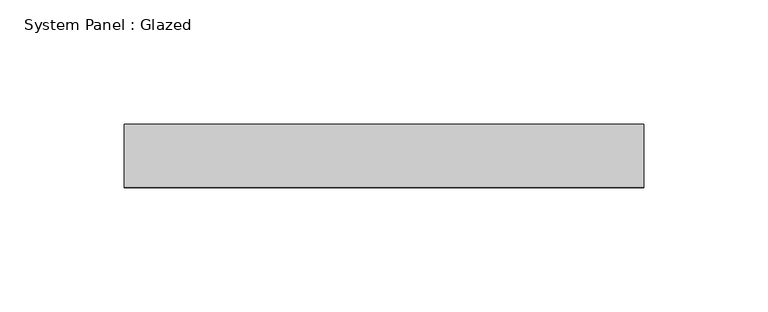
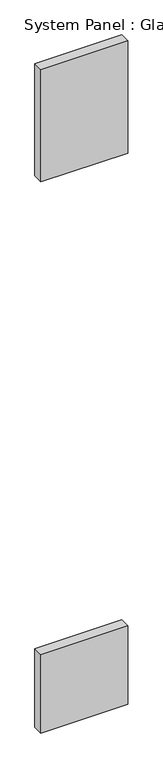
"""IFC4 building model written with IfcOpenShell, lengths in millimetres: plate geometry, System Panel : Glazed."""

from ifc_helpers import new_model, si_unit, frame, origin, origin_with_axes, place, context, project, spatial, polyline, outline, extrude, source, transform, mapped, element, save


def system_panel_glazed_c2730be0(model_context):
    return source(origin(), model_context, "Body", "SweptSolid", [
        extrude(outline(polyline([(104.775, 19.05), (-104.775, 19.05), (-104.775, 44.45), (104.775, 44.45), (104.775, 19.05)])), frame((0.0, 0.0, 1403.35), z_axis=(0.0, 0.0, 1.0), x_axis=(1.0, 0.0, 0.0)), (0.0, 0.0, 1.0), 285.75),
        extrude(outline(polyline([(104.775, 19.05), (-104.775, 19.05), (-104.775, 44.45), (104.775, 44.45), (104.775, 19.05)])), origin_with_axes(), (0.0, 0.0, 1.0), 199.39),
    ])


if __name__ == "__main__":
    model = new_model("IFC4")
    model_context = context("Model", 3, world=origin())
    ifc_project = project(units=[si_unit("LENGTHUNIT", "METRE", prefix="MILLI")], contexts=[model_context])
    site = spatial("IfcSite", under=ifc_project)
    building = spatial("IfcBuilding", under=site)
    placement = place(None, origin())
    system_panel_glazed_shape = system_panel_glazed_c2730be0(model_context)
    element("IfcPlate", 1, ObjectType="System Panel : Glazed", at=placement, inside=building, context=model_context, shape_type="MappedRepresentation", body=[
        mapped(system_panel_glazed_shape, transform((0.0, 0.0, 0.0), x_axis=(1.0, 0.0, 0.0), y_axis=(0.0, 1.0, 0.0), z_axis=(0.0, 0.0, 1.0))),
    ])
    save(model, "model.ifc")

# Revit data of these elements
# Type "System Panel : Glazed"
#   Construction Type Id = "GSP4R"
#   Analytic Construction = "1/8 in Pilkington single glazing"
#   Visual Light Transmittance = 0.9
#   Solar Heat Gain Coefficient = 0.86
#   Heat Transfer Coefficient (U) = 1.18115 BTU/(h·ft²·°F)
#   Define Thermal Properties by = 1
# Element 1 (IfcPlate, "System Panel : Glazed")
#   Materials on its faces: "Glass"
# Materials
#   "Glass": class "Glass", colour RGB 0 128 192, transparency 0.75, Description = "Soda Lime Glass", Cost = 0
